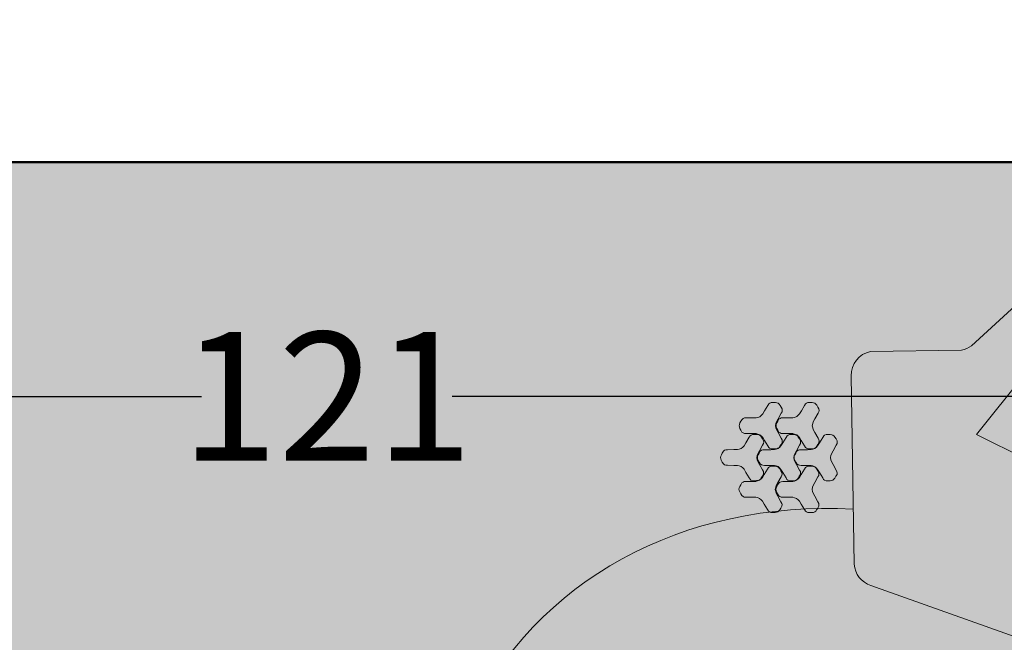
# Model space of a CAD drawing. Units: inches. Extents: x -466983 to 1020, y 324 to 318697.
# Tile 15 of 97: x 736 to 782, y 482 to 511. Entities that reach past the tile are written whole.
import ezdxf

# ---------------------------------------------------------------- set-up
doc = ezdxf.new("R2010")
doc.units = ezdxf.units.IN
doc.header["$MEASUREMENT"] = 0
for name, color, linetype, lineweight in [('A-ANNO-DIMS', 2, 'Continuous', 18), ('A-FLOR-PATT', 252, 'Continuous', 13), ('A-FURN', 8, 'Continuous', 18), ('A-WALL', 7, 'Continuous', 50)]:
    doc.layers.add(name, color=color, linetype=linetype, lineweight=lineweight)
doc.layers.add('K-Hatch', color=7, linetype='Continuous')
doc.styles.get("Standard").update_dxf_attribs({"font": 'arial.ttf'})
doc.dimstyles.get("Standard").update_dxf_attribs({"dimtxt": 6, "dimasz": 4, "dimexe": 3, "dimexo": 3, "dimgap": 0.09, "dimtad": 0, "dimtih": 1, "dimtoh": 1, "dimdec": 1, "dimzin": 0, "dimdsep": 46, "dimlunit": 3, "dimtxsty": 'Standard', "dimcen": 0.09, "dimadec": 0, "dimazin": 0, "dimtfac": 1, "dimtdec": 1, "dimtofl": 0, "dimtmove": 0, "dimatfit": 3, "dimfxl": 1, "dimtolj": 1, "dimtzin": 0, "dimarcsym": 0})

# ---------------------------------------------------------------- blocks, each defined once
blk = doc.blocks.new('CBV_05')
at = {"layer": 'K-Hatch'}
h = blk.add_hatch(color=256, dxfattribs=at)
h.dxf.hatch_style = 1
h.paths.add_polyline_path([(614, 437), (1251.4, 62.5), (1198.3, -263.2), (564.8, -9.8), (344.4, -5.5), (343.7, -629.7, 0.159768), (369.9, -672.6), (1020.5, -1025.6, 0.317347), (1135.5, -1017.7), (1739.5, -492.7, 0.378101), (1761.2, -362.2), (1507.4, -70.4, -0.119239), (1492.6, -25.8), (1499.5, 665.1, 0.256804), (1446.2, 745.4), (822.7, 1028.7, 0.297137), (714, 1018.3), (625, 963.6), (549.5, 1037.1), (186.8, 587.5), (-1106.2, 397.7), (-1098.6, 311.5), (-1098.4, 310.2)])
h.paths.add_polyline_path([(344.4, -5.5), (-1216.9, 24.6), (-1212.3, 260), (-1718.1, 162.7, 0.51466), (-1765.1, 50), (-1478.1, -479.5, 0.244482), (-1398.8, -526.6), (323.6, -658.2, 0.453292), (343.1, -629.8, 0.006511), (343.7, -631.8)])
h = blk.add_hatch(color=256, dxfattribs=at)
h.dxf.hatch_style = 1
h.paths.add_polyline_path([(614, 437), (-1211.5, 301.9), (-1212.3, 260), (-1216.9, 24.6), (564.8, -9.8), (1198.3, -263.2), (1251.4, 62.5)])
for p, q in [((186.8, 587.5), (549.5, 1037.1)), ((725.2, 866.1), (549.5, 1037.1)), ((517.5, 431), (725.2, 866.1)), ((-1106.2, 397.7), (186.8, 587.5)), ((-1211.5, 301.9), (614, 437)), ((614, 437), (1251.4, 62.5)), ((-1106.2, 397.7), (-1098.6, 311.5)), ((-1211.5, 301.9), (-1216.9, 24.6)), ((1251.4, 62.5), (1198.3, -263.2)), ((-1216.9, 24.6), (564.8, -9.8)), ((564.8, -9.8), (1198.3, -263.2))]:
    blk.add_line(p, q)
blk.add_lwpolyline([(1761.2, -362.2, -0.378101), (1739.5, -492.7), (1135.5, -1017.7, -0.317347), (1020.5, -1025.6), (369.9, -672.6, -0.159481), (343.2, -630.1, -0.449095), (323.6, -658.2), (-1398.8, -526.6, -0.244482), (-1478.1, -479.5), (-1765.1, 50, -0.51466), (-1718.1, 162.7), (-1212.3, 260), (-1211.5, 301.9), (-1098.4, 310.2), (-1106.2, 397.7), (186.8, 587.5), (549.5, 1037.1), (625, 963.6), (714, 1018.3, -0.297137), (822.7, 1028.7), (1446.2, 745.4, -0.256804), (1499.5, 665.1), (1492.6, -25.8, 0.119239), (1507.4, -70.4)], format="xyb", close=True)
for points in [[(369.9, -672.6), (1020.5, -1025.6, 0.317347), (1135.5, -1017.7), (1739.5, -492.7, 0.378101), (1761.2, -362.2), (1507.4, -70.4, -0.119239), (1492.6, -25.8), (1499.5, 665.1, 0.256804), (1446.2, 745.4), (822.7, 1028.7, 0.297137), (714, 1018.3), (625, 963.6)], [(-1212.3, 260), (-1718.1, 162.7, 0.51466), (-1765.1, 50), (-1478.1, -479.5, 0.244482), (-1398.8, -526.6), (323.6, -658.2)]]:
    blk.add_lwpolyline(points, format="xyb")
blk.add_lwpolyline([(344.4, -5.5), (343.7, -632.6)])
for centre, radius, start, end in [((422.2, -611.1), 80.7, 188.9571, 229.6497), ((320.9, -635.5), 22.9, 276.7908, 7.9615)]:
    blk.add_arc(centre, radius, start, end)
blk = doc.blocks.new('CBV_01')
for points in [[(-73.8, 112), (-73.8, 112), (-81.9, 116), (-89.2, 118.5), (-104, 120.4), (-130.7, 124), (-138.3, 125.2), (-142.9, 127.5), (-142.9, 127.5), (-147.8, 132.1), (-151.5, 140.5), (-154.6, 148.5), (-156.5, 154.6), (-156.5, 160.3), (-155.2, 165.8), (-152, 171.4), (-147.1, 178.5), (-141.6, 185.7), (-135.8, 189.1), (-135.8, 189.1), (-130.7, 190.3), (-123, 189.7), (-96.2, 187), (-81.4, 185.5), (-73.8, 186.3), (-64.6, 188.6), (-57.3, 193.4), (-51.5, 198.5), (-42.4, 210.3), (-25.9, 231.7), (-21, 237.7), (-16.7, 240.5), (-10.3, 242.5), (-1.2, 241.5), (7.3, 240.2), (13.6, 238.8), (18.5, 236), (22.6, 232.1), (25.8, 226.5), (29.5, 218.7), (33, 210.3), (33, 203.6), (31.5, 198.6), (27.2, 192.2), (11.5, 170.3), (2.7, 158.1), (-0.4, 151.2), (-3, 142.5), (-2.5, 133.4), (-1, 125.9), (4.7, 112.1), (15, 87.1), (17.7, 79.9), (18, 74.7), (16.5, 68.2), (11.1, 60.8), (5.7, 54.1), (1.4, 49.3), (-3.5, 46.5), (-8.9, 44.9), (-15.3, 44.9), (-23.9, 45.6), (-33, 46.8), (-38.8, 50.2), (-42.4, 53.9), (-45.8, 60.9), (-56.9, 85.4), (-63, 99.1), (-67.5, 105.3), (-73.8, 112)], [(81.4, 94.8), (81.4, 94.8), (73.2, 98.8), (66, 101.3), (51.2, 103.2), (24.5, 106.8), (16.9, 108), (12.3, 110.3), (12.2, 110.3), (7.3, 114.9), (3.6, 123.2), (0.5, 131.3), (-1.4, 137.4), (-1.4, 143.1), (-0.1, 148.6), (3.2, 154.1), (8.1, 161.2), (13.6, 168.5), (19.4, 171.8), (19.4, 171.8), (24.4, 173.1), (32.1, 172.5), (58.9, 169.8), (73.8, 168.3), (81.4, 169.1), (90.2, 171.1), (97.9, 176.2), (103.7, 181.2), (112.8, 193.1), (129.2, 214.5), (134.1, 220.5), (138.5, 223.3), (144.9, 225.3), (154, 224.3), (162.5, 223), (168.8, 221.6), (173.7, 218.8), (177.8, 214.9), (180.9, 209.3), (184.6, 201.5), (188.2, 193.1), (188.1, 186.4), (186.7, 181.4), (182.4, 175), (166.6, 153.1), (157.9, 140.9), (154.7, 134), (152.1, 125.3), (152.7, 116.2), (154.2, 108.7), (159.9, 94.8), (170.2, 69.9), (172.9, 62.7), (173.2, 57.5), (171.7, 51), (166.3, 43.6), (160.9, 36.8), (156.5, 32.1), (151.6, 29.3), (146.2, 27.7), (139.8, 27.7), (131.2, 28.4), (122.1, 29.5), (116.3, 32.9), (112.8, 36.7), (109.4, 43.7), (98.3, 68.2), (92.1, 81.9), (87.7, 88.1), (81.4, 94.8)], [(-158.4, 63.7), (-150.8, 68.7), (-145, 73.8), (-135.9, 85.6), (-119.4, 107), (-114.5, 113), (-110.2, 115.8), (-103.8, 117.8), (-94.7, 116.8), (-86.2, 115.5), (-79.9, 114.1), (-75, 111.3), (-70.9, 107.4), (-67.7, 101.8), (-64, 94), (-60.5, 85.6), (-60.5, 78.9), (-62, 73.9), (-66.3, 67.5), (-82, 45.6), (-90.8, 33.5), (-93.9, 26.5), (-96.5, 17.8), (-96, 8.7), (-94.5, 1.2), (-88.8, -12.6), (-78.5, -37.6), (-75.8, -44.8), (-75.5, -50), (-77, -56.5), (-82.4, -63.9), (-87.8, -70.6), (-92.1, -75.3), (-97, -78.2), (-102.4, -79.8), (-108.8, -79.7), (-117.4, -79.1), (-126.5, -77.9), (-132.3, -74.5), (-135.9, -70.8), (-139.3, -63.8), (-150.4, -39.2), (-156.5, -25.6), (-161, -19.4), (-167.3, -12.7), (-175.4, -8.7), (-182.7, -6.2), (-197.5, -4.2), (-224.2, -0.7), (-231.8, 0.5), (-236.4, 2.9), (-236.4, 2.9), (-241.3, 7.4), (-245, 15.8), (-248.1, 23.8), (-250, 29.9), (-250, 35.6), (-248.7, 41.1), (-245.5, 46.7), (-240.6, 53.8), (-235.1, 61.1), (-229.3, 64.4), (-229.3, 64.4), (-224.2, 65.6), (-216.5, 65), (-189.7, 62.4), (-174.9, 60.9), (-167.3, 61.6), (-158.4, 63.7), (-158.4, 63.7)], [(-12.1, -31.2), (-12.1, -31.2), (-20.3, -27.2), (-27.5, -24.7), (-42.3, -22.7), (-69, -19.2), (-76.6, -18), (-81.2, -15.6), (-81.2, -15.6), (-86.2, -11.1), (-89.8, -2.7), (-93, 5.3), (-94.9, 11.4), (-94.9, 17.1), (-93.6, 22.6), (-90.3, 28.2), (-85.4, 35.3), (-79.9, 42.5), (-74.1, 45.9), (-74.1, 45.9), (-69, 47.1), (-61.4, 46.5), (-34.6, 43.8), (-19.7, 42.3), (-12.1, 43.1), (-3.3, 45.2), (4.4, 50.2), (10.2, 55.3), (19.3, 67.1), (35.7, 88.5), (40.6, 94.5), (45, 97.3), (51.4, 99.3), (60.5, 98.3), (69, 97), (75.3, 95.6), (80.2, 92.8), (84.3, 88.9), (87.4, 83.3), (91.2, 75.5), (94.7, 67.1), (94.7, 60.4), (93.2, 55.4), (88.9, 49), (73.1, 27.1), (64.4, 14.9), (61.3, 8), (58.6, -0.7), (59.2, -9.8), (60.7, -17.3), (66.4, -31.1), (76.7, -56.1), (79.4, -63.3), (79.7, -68.5), (78.2, -75), (72.8, -82.4), (67.4, -89.1), (63, -93.8), (58.2, -96.7), (52.7, -98.3), (46.3, -98.2), (37.7, -97.6), (28.7, -96.4), (22.9, -93), (19.3, -89.3), (15.9, -82.3), (4.8, -57.7), (-1.4, -44.1), (-5.8, -37.9), (-12.1, -31.2)], [(152, 27.3), (159.7, 32.4), (165.5, 37.4), (174.6, 49.3), (191, 70.7), (195.9, 76.6), (200.3, 79.5), (206.7, 81.5), (215.8, 80.5), (224.3, 79.2), (230.6, 77.7), (235.5, 74.9), (239.6, 71.1), (242.7, 65.5), (246.5, 57.7), (250, 49.3), (250, 42.5), (248.5, 37.6), (244.2, 31.2), (228.4, 9.3), (219.7, -2.9), (216.6, -9.9), (213.9, -18.6), (214.5, -27.6), (216, -35.1), (221.7, -49), (232, -73.9), (234.7, -81.1), (235, -86.3), (233.5, -92.9), (228.1, -100.2), (222.7, -107), (218.3, -111.7), (213.5, -114.5), (208.1, -116.1), (201.6, -116.1), (193, -115.4), (184, -114.3), (178.2, -110.9), (174.6, -107.1), (171.2, -100.2), (160.1, -75.6), (153.9, -62), (149.5, -55.7), (143.2, -49), (135, -45), (127.8, -42.5), (113, -40.6), (86.3, -37.1), (78.7, -35.8), (74.1, -33.5), (74.1, -33.5), (69.1, -28.9), (65.5, -20.6), (62.3, -12.5), (60.5, -6.4), (60.5, -0.7), (61.8, 4.8), (65, 10.3), (69.9, 17.4), (75.4, 24.7), (81.2, 28), (81.2, 28), (86.3, 29.2), (93.9, 28.7), (120.7, 26), (135.6, 24.5), (143.2, 25.3), (152.1, 27.3), (152, 27.3)], [(-105, -156.9), (-105, -156.9), (-113.1, -152.9), (-120.3, -150.4), (-135.1, -148.4), (-161.8, -144.9), (-169.4, -143.7), (-174.1, -141.3), (-174.1, -141.3), (-179, -136.8), (-182.7, -128.4), (-185.8, -120.4), (-187.7, -114.3), (-187.7, -108.6), (-186.4, -103.1), (-183.1, -97.5), (-178.3, -90.4), (-172.8, -83.2), (-166.9, -79.8), (-166.9, -79.8), (-161.9, -78.6), (-154.2, -79.2), (-127.4, -81.9), (-112.5, -83.4), (-104.9, -82.6), (-96.1, -80.5), (-88.4, -75.5), (-82.7, -70.4), (-73.5, -58.6), (-57.1, -37.2), (-52.2, -31.2), (-47.9, -28.4), (-41.4, -26.4), (-32.4, -27.4), (-23.8, -28.7), (-17.6, -30.1), (-12.7, -32.9), (-8.6, -36.8), (-5.4, -42.4), (-1.7, -50.2), (1.9, -58.6), (1.8, -65.3), (0.3, -70.3), (-4, -76.7), (-19.7, -98.6), (-28.4, -110.8), (-31.6, -117.7), (-34.2, -126.4), (-33.6, -135.5), (-32.2, -143), (-26.5, -156.8), (-16.2, -181.8), (-13.4, -189), (-13.1, -194.2), (-14.6, -200.7), (-20, -208.1), (-25.4, -214.8), (-29.8, -219.5), (-34.7, -222.4), (-40.1, -224), (-46.5, -223.9), (-55.1, -223.3), (-64.2, -222.1), (-70, -218.7), (-73.6, -215), (-76.9, -208), (-88, -183.4), (-94.2, -169.8), (-98.7, -163.6), (-105, -156.9)], [(59.1, -99), (66.7, -94), (72.5, -88.9), (81.6, -77.1), (98.1, -55.7), (102.9, -49.7), (107.3, -46.9), (113.7, -44.9), (122.8, -45.9), (131.3, -47.2), (137.6, -48.6), (142.5, -51.4), (146.6, -55.3), (149.8, -60.9), (153.5, -68.7), (157, -77.1), (157, -83.8), (155.5, -88.8), (151.2, -95.2), (135.5, -117.1), (126.7, -129.3), (123.6, -136.2), (121, -144.9), (121.5, -154), (123, -161.5), (128.7, -175.3), (139, -200.3), (141.7, -207.5), (142, -212.7), (140.5, -219.2), (135.1, -226.6), (129.7, -233.3), (125.4, -238.1), (120.5, -240.9), (115.1, -242.5), (108.6, -242.5), (100, -241.8), (91, -240.6), (85.2, -237.2), (81.6, -233.5), (78.2, -226.5), (67.1, -202), (61, -188.3), (56.5, -182.1), (50.2, -175.4), (42.1, -171.4), (34.8, -168.9), (20, -167), (-6.7, -163.4), (-14.3, -162.2), (-18.9, -159.9), (-18.9, -159.9), (-23.8, -155.3), (-27.5, -146.9), (-30.6, -138.9), (-32.5, -132.8), (-32.5, -127.1), (-31.2, -121.6), (-28, -116), (-23.1, -108.9), (-17.6, -101.7), (-11.8, -98.3), (-11.8, -98.3), (-6.7, -97.1), (1, -97.7), (27.8, -100.4), (42.6, -101.9), (50.2, -101.1), (59.1, -99), (59.1, -99)]]:
    blk.add_lwpolyline(points)
blk = doc.blocks.new('Garden Sofa')
at = {"extrusion": (0, 0, -1)}
blk.add_ellipse((2450.434, 828.917), major_axis=(18.681, -14.923), ratio=0.833526, start_param=9.234639, end_param=10.284819, dxfattribs=at)
at = {"xscale": -0.0109740885734132, "yscale": 0.0109740885734132, "zscale": 0.0109740885734132}
for name, p, rotation in [('CBV_05', (2464.355, 846.083), 311.9356943688126), ('CBV_01', (2444.425, 852.692), 293.2804071400473)]:
    blk.add_blockref(name, p, dxfattribs=dict(at, rotation=rotation))
blk = doc.blocks.new('*D70')
at = {"layer": 'A-ANNO-DIMS', "color": 0, "lineweight": -2, "transparency": 16777216}
for p, q in [((689.806, 508.686), (689.806, 490.005)), ((810.968, 508.686), (810.968, 490.005)), ((693.806, 493.005), (744.53, 493.005)), ((806.968, 493.005), (756.244, 493.005))]:
    blk.add_line(p, q, dxfattribs=at)
at = {"layer": 'A-ANNO-DIMS', "color": 0, "transparency": 16777216}
for points in [[(693.806, 493.671), (693.806, 492.338), (689.806, 493.005)], [(806.968, 493.671), (806.968, 492.338), (810.968, 493.005)]]:
    blk.add_solid(points, dxfattribs=at)
at = {"layer": 'Defpoints', "color": 0, "transparency": 16777216}
for p in [(689.806, 511.686), (810.968, 511.686), (810.968, 493.005)]:
    blk.add_point(p, dxfattribs=at)
at = {"layer": 'A-ANNO-DIMS', "color": 0, "transparency": 16777216, "insert": (750.387, 493.005), "char_height": 6, "attachment_point": 5}
blk.add_mtext('\\A1;121', dxfattribs=at)
blk = doc.blocks.new('*D113')
at = {"layer": 'A-ANNO-DIMS', "color": 0, "lineweight": -2, "transparency": 16777216}
for p, q in [((704.71, 504.652), (709.525, 509.413)), ((710.204, 504.46), (736.319, 478.049)), ((736.45, 472.553), (741.265, 477.314)), ((739.132, 475.204), (741.944, 472.36)), ((741.944, 472.36), (745.944, 472.36))]:
    blk.add_line(p, q, dxfattribs=at)
at = {"layer": 'A-ANNO-DIMS', "color": 0, "transparency": 16777216}
for points in [[(710.678, 504.928), (709.73, 503.991), (707.392, 507.304)], [(736.794, 478.517), (735.845, 477.58), (739.132, 475.204)]]:
    blk.add_solid(points, dxfattribs=at)
at = {"layer": 'Defpoints', "color": 0, "transparency": 16777216}
for p in [(702.577, 502.543), (739.132, 475.204), (734.317, 470.443)]:
    blk.add_point(p, dxfattribs=at)
at = {"layer": 'A-ANNO-DIMS', "color": 0, "transparency": 16777216, "insert": (783.502, 472.36), "char_height": 6, "attachment_point": 5}
blk.add_mtext('\\A1;TEA TABLE SET 45', dxfattribs=at)

msp = doc.modelspace()

# ---------------------------------------------------------------- hatches: boundary and pattern name
at = {"layer": 'A-FLOR-PATT', "transparency": 33554661}
h = msp.add_hatch(color=256, dxfattribs=at)
h.dxf.hatch_style = 1
h.set_gradient(color1=(19, 155, 72), color2=(0, 107, 0), name='CYLINDER')
h.paths.add_polyline_path([(813.806, 503.938), (730.806, 503.938), (730.806, 424.938), (612.806, 424.938), (612.806, 415.938), (442.806, 415.938), (442.806, 368.938), (813.806, 368.938)])
h.paths.add_polyline_path([(771.796, 407.07), (783.796, 407.07), (783.796, 371.07), (771.796, 371.07)], flags=16)
h.paths.add_polyline_path([(755.796, 407.07), (755.796, 371.07), (743.796, 371.07), (743.796, 407.07)], flags=16)
h.paths.add_polyline_path([(769.796, 404.07), (769.796, 374.07), (757.796, 374.07), (757.796, 404.07)], flags=16)
h.paths.add_polyline_path([(785.796, 404.07), (797.796, 404.07), (797.796, 374.07), (785.796, 374.07)], flags=16)
h.paths.add_polyline_path([(741.796, 404.07), (741.796, 374.07), (729.796, 374.07), (729.796, 404.07)], flags=16)
h.paths.add_polyline_path([(799.796, 407.07), (811.796, 407.07), (811.796, 371.07), (799.796, 371.07)], flags=16)
h.paths.add_polyline_path([(727.796, 407.07), (727.796, 371.07), (715.796, 371.07), (715.796, 407.07)], flags=16)
h.paths.add_polyline_path([(713.796, 404.07), (713.796, 374.07), (701.796, 374.07), (701.796, 404.07)], flags=16)
h.paths.add_polyline_path([(699.796, 407.07), (699.796, 371.07), (687.796, 371.07), (687.796, 407.07)], flags=16)
h.paths.add_polyline_path([(685.796, 404.07), (685.796, 374.07), (673.796, 374.07), (673.796, 404.07)], flags=16)
h.paths.add_polyline_path([(671.796, 407.07), (671.796, 371.07), (659.796, 371.07), (659.796, 407.07)], flags=16)
h.paths.add_polyline_path([(657.796, 404.07), (657.796, 374.07), (645.796, 374.07), (645.796, 404.07)], flags=16)
h.paths.add_polyline_path([(643.796, 407.07), (643.796, 371.07), (631.796, 371.07), (631.796, 407.07)], flags=16)
h.paths.add_polyline_path([(629.796, 404.07), (629.796, 374.07), (617.796, 374.07), (617.796, 404.07)], flags=16)
h.paths.add_polyline_path([(615.796, 407.07), (615.796, 371.07), (603.796, 371.07), (603.796, 407.07)], flags=16)
h.paths.add_polyline_path([(601.796, 404.07), (601.796, 374.07), (589.796, 374.07), (589.796, 404.07)], flags=16)
at = {"layer": 'A-FLOR-PATT'}
h = msp.add_hatch(dxfattribs=at)
h.set_pattern_fill('GRASS', color=256, scale=6)
h.set_pattern_definition([(90, (-1212.4137, -290.035), (-4.242641, 4.242641), [1.125, -7.360281]), (45, (-1212.4137, -290.035), (-4.24264, 4.24264), [1.125, -4.875]), (135, (-1212.4137, -290.035), (-4.24264, -4.24264), [1.125, -4.875])])
h.paths.add_polyline_path([(813.806, 503.938), (730.806, 503.938), (730.806, 424.938), (612.806, 424.938), (612.806, 415.938), (442.806, 415.938), (442.806, 368.938), (813.806, 368.938)])
h.paths.add_polyline_path([(589.796, 404.07), (601.796, 404.07), (601.796, 374.07), (589.796, 374.07)], flags=16)
h.paths.add_polyline_path([(603.796, 407.07), (615.796, 407.07), (615.796, 371.07), (603.796, 371.07)], flags=16)
h.paths.add_polyline_path([(617.796, 404.07), (629.796, 404.07), (629.796, 374.07), (617.796, 374.07)], flags=16)
h.paths.add_polyline_path([(631.796, 407.07), (643.796, 407.07), (643.796, 371.07), (631.796, 371.07)], flags=16)
h.paths.add_polyline_path([(645.796, 404.07), (657.796, 404.07), (657.796, 374.07), (645.796, 374.07)], flags=16)
h.paths.add_polyline_path([(659.796, 407.07), (671.796, 407.07), (671.796, 371.07), (659.796, 371.07)], flags=16)
h.paths.add_polyline_path([(673.796, 404.07), (685.796, 404.07), (685.796, 374.07), (673.796, 374.07)], flags=16)
h.paths.add_polyline_path([(687.796, 407.07), (699.796, 407.07), (699.796, 371.07), (687.796, 371.07)], flags=16)
h.paths.add_polyline_path([(701.796, 404.07), (713.796, 404.07), (713.796, 374.07), (701.796, 374.07)], flags=16)
h.paths.add_polyline_path([(715.796, 407.07), (727.796, 407.07), (727.796, 371.07), (715.796, 371.07)], flags=16)
h.paths.add_polyline_path([(729.796, 404.07), (741.796, 404.07), (741.796, 374.07), (729.796, 374.07)], flags=16)
h.paths.add_polyline_path([(743.796, 407.07), (755.796, 407.07), (755.796, 371.07), (743.796, 371.07)], flags=16)
h.paths.add_polyline_path([(757.796, 404.07), (769.796, 404.07), (769.796, 374.07), (757.796, 374.07)], flags=16)
h.paths.add_polyline_path([(771.796, 407.07), (783.796, 407.07), (783.796, 371.07), (771.796, 371.07)], flags=16)
h.paths.add_polyline_path([(785.796, 404.07), (797.796, 404.07), (797.796, 374.07), (785.796, 374.07)], flags=16)
h.paths.add_polyline_path([(799.796, 407.07), (811.796, 407.07), (811.796, 371.07), (799.796, 371.07)], flags=16)

# ---------------------------------------------------------------- linework, layer by layer
at = {"layer": 'A-WALL'}
msp.add_line((813.806, 503.938), (618.806, 503.938), dxfattribs=at)

# ---------------------------------------------------------------- block references
at = {"layer": 'A-FURN'}
msp.add_blockref('Garden Sofa', (-1672.7, -362.711), dxfattribs=at)

# ---------------------------------------------------------------- dimensions: what is measured, and where the dimension line sits
at = {"layer": 'A-ANNO-DIMS'}
dim = msp.add_linear_dim(base=(810.968, 493.005), p1=(689.806, 511.686), p2=(810.968, 511.686), dimstyle='Standard', override={"dimdec": 0, "dimlfac": 1, "dimrnd": 0, "dimzin": 0, "dimdsep": 46, "dimlunit": 2}, dxfattribs=at)
dim.commit()
dim.dimension.update_dxf_attribs({"geometry": '*D70', "text_midpoint": (750.387, 493.005)})
dim = msp.add_linear_dim(base=(739.132, 475.204), p1=(702.577, 502.543), p2=(734.317, 470.443), angle=314.6775, text='TEA TABLE SET <>', dimstyle='Standard', override={"dimdec": 0, "dimlfac": 1, "dimrnd": 0, "dimzin": 0, "dimdsep": 46, "dimlunit": 2}, dxfattribs=at)
dim.commit()
dim.dimension.update_dxf_attribs({"geometry": '*D113', "text_midpoint": (783.502, 472.36)})

doc.saveas('drawing.dxf')
